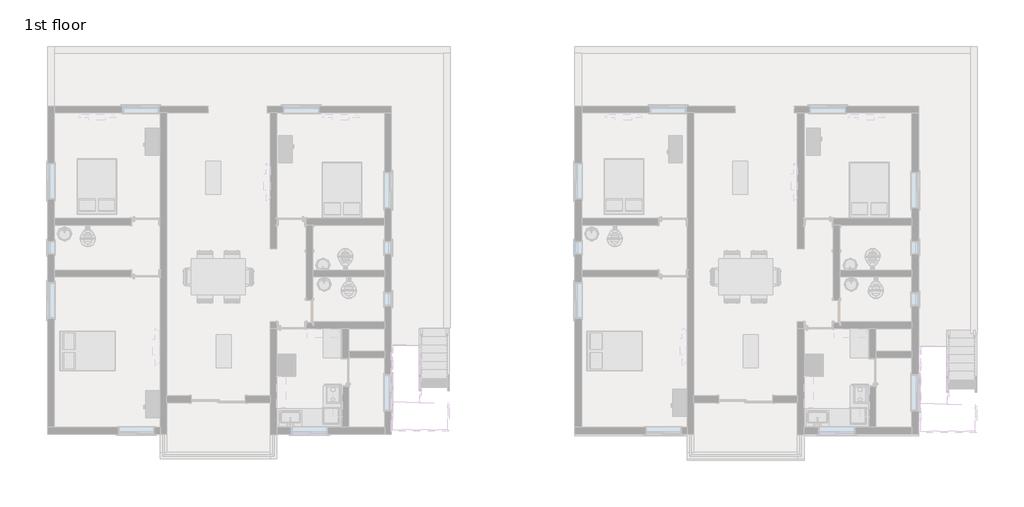
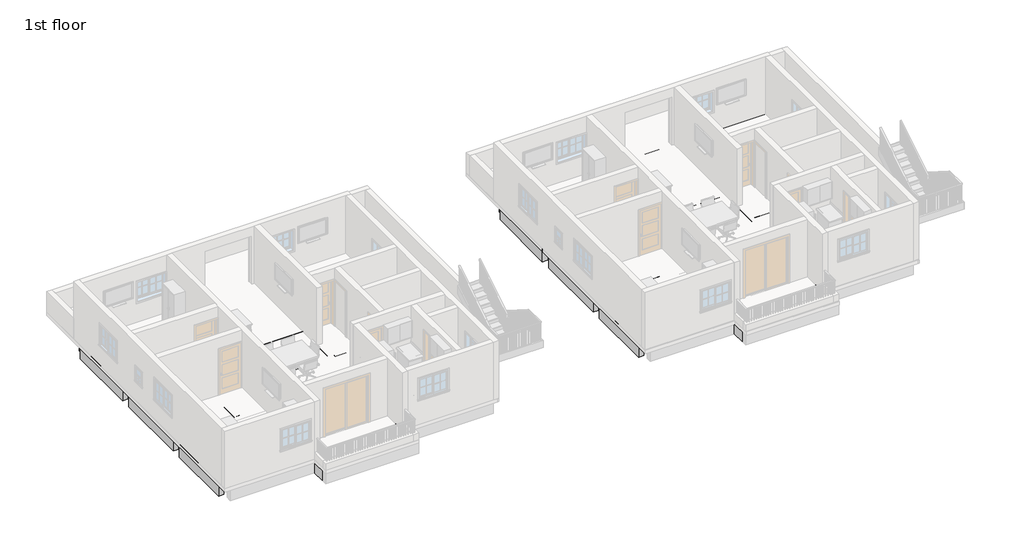
# One storey, part 3 of 8: 30 beams.
"""IFC4 building model written with IfcOpenShell, lengths in millimetres."""

from ifc_helpers import new_model, si_unit, frame, origin, place, context, project, spatial, polyline, outline, extrude, faceted_brep, element, save

model = new_model("IFC4")

# Units and contexts
model_context = context("Model", 3, world=origin())
ifc_project = project(units=[si_unit("LENGTHUNIT", "METRE", prefix="MILLI")], contexts=[model_context])

# Site, building, storey
site = spatial("IfcSite", under=ifc_project)
building = spatial("IfcBuilding", under=site)
storey = spatial("IfcBuildingStorey", under=building, Name="1st floor", Elevation=3810.0)

# Beams
placement = place(None, origin())
element("IfcBeam", 1, ObjectType="Concrete-Rectangular Beam", at=placement, inside=storey, context=model_context, shape_type="Brep", body=[
    faceted_brep([(-16300.5993763, -4148.1064015, 3810.0), (-16071.9993763, -4148.1064015, 3810.0), (-16071.9993763, -1252.5064015, 3810.0), (-16300.5993763, -1252.5064015, 3810.0), (-16300.5993763, -4148.1064015, 3200.4), (-16300.5993763, -1252.5064015, 3200.4), (-16071.9993763, -4148.1064015, 3200.4), (-16071.9993763, -1252.5064015, 3200.4)], [[[0, 1, 2, 3]], [[4, 0, 3, 5]], [[6, 4, 5, 7]], [[1, 6, 7, 2]], [[1, 0, 4, 6]], [[3, 2, 7, 5]]]),
    faceted_brep([(-16300.5993763, 6062.6935985, 3810.0), (-16071.9993763, 6062.6935985, 3810.0), (-16071.9993763, 6062.6935985, 3200.4), (-16300.5993763, 6062.6935985, 3200.4), (-16071.9993763, 2938.4935985, 3810.0), (-16300.5993763, 2938.4935985, 3810.0), (-16300.5993763, 2938.4935985, 3200.4), (-16071.9993763, 2938.4935985, 3200.4)], [[[0, 1, 2, 3]], [[4, 5, 6, 7]], [[1, 0, 5, 4]], [[0, 3, 6, 5]], [[3, 2, 7, 6]], [[2, 1, 4, 7]]]),
    faceted_brep([(-16300.5993763, 2481.2935985, 3810.0), (-16071.9993763, 2481.2935985, 3810.0), (-16071.9993763, 2481.2935985, 3200.4), (-16300.5993763, 2481.2935985, 3200.4), (-16071.9993763, -795.3064015, 3810.0), (-16300.5993763, -795.3064015, 3810.0), (-16300.5993763, -795.3064015, 3200.4), (-16071.9993763, -795.3064015, 3200.4), (-16071.9993763, 728.6935985, 3810.0), (-16071.9993763, 957.2935985, 3810.0), (-16071.9993763, 957.2935985, 3200.4), (-16071.9993763, 728.6935985, 3200.4)], [[[0, 1, 2, 3]], [[4, 5, 6, 7]], [[1, 0, 5, 4, 8, 9]], [[0, 3, 6, 5]], [[3, 2, 10, 11, 7, 6]], [[2, 1, 9, 8, 4, 7, 11, 10]]]),
])
element("IfcBeam", 2, ObjectType="Concrete-Rectangular Beam", at=placement, inside=storey, context=model_context, shape_type="SweptSolid", body=[
    extrude(outline(polyline([(-16071.9993763, 6291.2935985), (-16071.9993763, 6519.8935985), (-12490.5993763, 6519.8935985), (-12490.5993763, 6291.2935985), (-16071.9993763, 6291.2935985)])), frame((0.0, 0.0, 3200.4), z_axis=(0.0, 0.0, 1.0), x_axis=(1.0, 0.0, 0.0)), (0.0, 0.0, 1.0), 609.6),
    extrude(outline(polyline([(-4870.5993763, 6519.8935985), (-4870.5993763, 6291.2935985), (-8528.1993763, 6291.2935985), (-8528.1993763, 6519.8935985), (-4870.5993763, 6519.8935985)])), frame((0.0, 0.0, 3200.4), z_axis=(0.0, 0.0, 1.0), x_axis=(1.0, 0.0, 0.0)), (0.0, 0.0, 1.0), 609.6),
    extrude(outline(polyline([(-12261.9993763, 6291.2935985), (-12261.9993763, 6519.8935985), (-8756.7993763, 6519.8935985), (-8756.7993763, 6291.2935985), (-12261.9993763, 6291.2935985)])), frame((0.0, 0.0, 3200.4), z_axis=(0.0, 0.0, 1.0), x_axis=(1.0, 0.0, 0.0)), (0.0, 0.0, 1.0), 609.6),
])
element("IfcBeam", 3, ObjectType="Concrete-Rectangular Beam", at=placement, inside=storey, context=model_context, shape_type="Brep", body=[
    faceted_brep([(-12261.9993763, -4605.3064015, 3810.0), (-12490.5993763, -4605.3064015, 3810.0), (-12490.5993763, -5214.9064015, 3810.0), (-12261.9993763, -5214.9064015, 3810.0), (-12490.5993763, -4605.3064015, 3200.4), (-12490.5993763, -5214.9064015, 3200.4), (-12261.9993763, -4605.3064015, 3200.4), (-12261.9993763, -5214.9064015, 3200.4)], [[[0, 1, 2, 3]], [[1, 4, 5, 2]], [[4, 6, 7, 5]], [[6, 0, 3, 7]], [[1, 0, 6, 4]], [[3, 2, 5, 7]]]),
    faceted_brep([(-12490.5993763, 6062.6935985, 3810.0), (-12261.9993763, 6062.6935985, 3810.0), (-12261.9993763, 6062.6935985, 3200.4), (-12490.5993763, 6062.6935985, 3200.4), (-12261.9993763, 2938.4935985, 3810.0), (-12490.5993763, 2938.4935985, 3810.0), (-12490.5993763, 2938.4935985, 3200.4), (-12261.9993763, 2938.4935985, 3200.4)], [[[0, 1, 2, 3]], [[4, 5, 6, 7]], [[1, 0, 5, 4]], [[0, 3, 6, 5]], [[3, 2, 7, 6]], [[2, 1, 4, 7]]]),
    faceted_brep([(-12261.9993763, -4148.1064015, 3810.0), (-12490.5993763, -4148.1064015, 3810.0), (-12490.5993763, -4148.1064015, 3200.4), (-12261.9993763, -4148.1064015, 3200.4), (-12490.5993763, -1252.5064015, 3810.0), (-12261.9993763, -1252.5064015, 3810.0), (-12261.9993763, -1252.5064015, 3200.4), (-12490.5993763, -1252.5064015, 3200.4), (-12261.9993763, -3538.5064015, 3810.0), (-12261.9993763, -3309.9064015, 3810.0), (-12261.9993763, -3309.9064015, 3200.4), (-12261.9993763, -3538.5064015, 3200.4)], [[[0, 1, 2, 3]], [[4, 5, 6, 7]], [[1, 0, 8, 9, 5, 4]], [[2, 1, 4, 7]], [[3, 2, 7, 6, 10, 11]], [[0, 3, 11, 10, 6, 5, 9, 8]]]),
    faceted_brep([(-12490.5993763, 2481.2935985, 3810.0), (-12261.9993763, 2481.2935985, 3810.0), (-12261.9993763, 2481.2935985, 3200.4), (-12490.5993763, 2481.2935985, 3200.4), (-12261.9993763, -795.3064015, 3810.0), (-12490.5993763, -795.3064015, 3810.0), (-12490.5993763, -795.3064015, 3200.4), (-12261.9993763, -795.3064015, 3200.4), (-12490.5993763, 957.2935985, 3810.0), (-12490.5993763, 728.6935985, 3810.0), (-12261.9993763, 728.6935985, 3810.0), (-12261.9993763, 957.2935985, 3810.0), (-12490.5993763, 957.2935985, 3200.4), (-12490.5993763, 728.6935985, 3200.4), (-12261.9993763, 957.2935985, 3200.4), (-12261.9993763, 728.6935985, 3200.4)], [[[0, 1, 2, 3]], [[4, 5, 6, 7]], [[1, 0, 8, 9, 5, 4, 10, 11]], [[0, 3, 12, 13, 6, 5, 9, 8]], [[3, 2, 14, 15, 7, 6, 13, 12]], [[2, 1, 11, 10, 4, 7, 15, 14]]]),
])
element("IfcBeam", 4, ObjectType="Concrete-Rectangular Beam", at=placement, inside=storey, context=model_context, shape_type="Brep", body=[
    faceted_brep([(-8528.1993763, 6062.6935985, 3810.0), (-8756.7993763, 6062.6935985, 3810.0), (-8756.7993763, 2938.4935985, 3810.0), (-8528.1993763, 2938.4935985, 3810.0), (-8528.1993763, 6062.6935985, 3200.4), (-8528.1993763, 2938.4935985, 3200.4), (-8756.7993763, 6062.6935985, 3200.4), (-8756.7993763, 2938.4935985, 3200.4)], [[[0, 1, 2, 3]], [[4, 0, 3, 5]], [[6, 4, 5, 7]], [[1, 6, 7, 2]], [[1, 0, 4, 6]], [[3, 2, 7, 5]]]),
    faceted_brep([(-8528.1993763, -5214.9064015, 3810.0), (-8756.7993763, -5214.9064015, 3810.0), (-8756.7993763, -5214.9064015, 3200.4), (-8528.1993763, -5214.9064015, 3200.4), (-8756.7993763, -4605.3064015, 3810.0), (-8528.1993763, -4605.3064015, 3810.0), (-8528.1993763, -4605.3064015, 3200.4), (-8756.7993763, -4605.3064015, 3200.4)], [[[0, 1, 2, 3]], [[4, 5, 6, 7]], [[1, 0, 5, 4]], [[0, 3, 6, 5]], [[3, 2, 7, 6]], [[2, 1, 4, 7]]]),
    faceted_brep([(-8528.1993763, -4148.1064015, 3810.0), (-8756.7993763, -4148.1064015, 3810.0), (-8756.7993763, -4148.1064015, 3200.4), (-8528.1993763, -4148.1064015, 3200.4), (-8756.7993763, -1252.5064015, 3810.0), (-8528.1993763, -1252.5064015, 3810.0), (-8528.1993763, -1252.5064015, 3200.4), (-8756.7993763, -1252.5064015, 3200.4), (-8756.7993763, -3309.9064015, 3810.0), (-8756.7993763, -3538.5064015, 3810.0), (-8756.7993763, -3538.5064015, 3200.4), (-8756.7993763, -3309.9064015, 3200.4)], [[[0, 1, 2, 3]], [[4, 5, 6, 7]], [[1, 0, 5, 4, 8, 9]], [[0, 3, 6, 5]], [[3, 2, 10, 11, 7, 6]], [[2, 1, 9, 8, 4, 7, 11, 10]]]),
    faceted_brep([(-8756.7993763, 2481.2935985, 3810.0), (-8528.1993763, 2481.2935985, 3810.0), (-8528.1993763, 2481.2935985, 3200.4), (-8756.7993763, 2481.2935985, 3200.4), (-8756.7993763, 957.2935985, 3810.0), (-8756.7993763, 728.6935985, 3810.0), (-8756.7993763, -795.3064015, 3810.0), (-8528.1993763, -795.3064015, 3810.0), (-8528.1993763, 728.6935985, 3810.0), (-8528.1993763, 957.2935985, 3810.0), (-8528.1993763, -795.3064015, 3200.4), (-8528.1993763, 728.6935985, 3200.4), (-8528.1993763, 957.2935985, 3200.4), (-8756.7993763, -795.3064015, 3200.4), (-8756.7993763, 728.6935985, 3200.4), (-8756.7993763, 957.2935985, 3200.4)], [[[0, 1, 2, 3]], [[1, 0, 4, 5, 6, 7, 8, 9]], [[2, 1, 9, 8, 7, 10, 11, 12]], [[3, 2, 12, 11, 10, 13, 14, 15]], [[0, 3, 15, 14, 13, 6, 5, 4]], [[7, 6, 13, 10]]]),
])
element("IfcBeam", 5, ObjectType="Concrete-Rectangular Beam", at=placement, inside=storey, context=model_context, shape_type="Brep", body=[
    faceted_brep([(-4870.5993763, -4148.1064015, 3810.0), (-4641.9993763, -4148.1064015, 3810.0), (-4641.9993763, -1023.9064015, 3810.0), (-4870.5993763, -1023.9064015, 3810.0), (-4870.5993763, -1785.9064015, 3810.0), (-4870.5993763, -2014.5064015, 3810.0), (-4870.5993763, -4148.1064015, 3200.4), (-4870.5993763, -1023.9064015, 3200.4), (-4870.5993763, -1785.9064015, 3200.4), (-4870.5993763, -2014.5064015, 3200.4), (-4641.9993763, -4148.1064015, 3200.4), (-4641.9993763, -1023.9064015, 3200.4)], [[[0, 1, 2, 3, 4, 5]], [[6, 0, 5, 4, 3, 7, 8, 9]], [[10, 6, 9, 8, 7, 11]], [[1, 10, 11, 2]], [[1, 0, 6, 10]], [[3, 2, 11, 7]]]),
    faceted_brep([(-4870.5993763, 6062.6935985, 3810.0), (-4641.9993763, 6062.6935985, 3810.0), (-4641.9993763, 6062.6935985, 3200.4), (-4870.5993763, 6062.6935985, 3200.4), (-4641.9993763, 2938.4935985, 3810.0), (-4870.5993763, 2938.4935985, 3810.0), (-4870.5993763, 2938.4935985, 3200.4), (-4641.9993763, 2938.4935985, 3200.4)], [[[0, 1, 2, 3]], [[4, 5, 6, 7]], [[1, 0, 5, 4]], [[0, 3, 6, 5]], [[3, 2, 7, 6]], [[2, 1, 4, 7]]]),
    faceted_brep([(-4870.5993763, 2481.2935985, 3810.0), (-4641.9993763, 2481.2935985, 3810.0), (-4641.9993763, 2481.2935985, 3200.4), (-4870.5993763, 2481.2935985, 3200.4), (-4641.9993763, -566.7064015, 3810.0), (-4870.5993763, -566.7064015, 3810.0), (-4870.5993763, -566.7064015, 3200.4), (-4641.9993763, -566.7064015, 3200.4), (-4870.5993763, 957.2935985, 3810.0), (-4870.5993763, 728.6935985, 3810.0), (-4870.5993763, 957.2935985, 3200.4), (-4870.5993763, 728.6935985, 3200.4)], [[[0, 1, 2, 3]], [[4, 5, 6, 7]], [[1, 0, 8, 9, 5, 4]], [[0, 3, 10, 11, 6, 5, 9, 8]], [[3, 2, 7, 6, 11, 10]], [[2, 1, 4, 7]]]),
])
element("IfcBeam", 6, ObjectType="Concrete-Rectangular Beam", at=placement, inside=storey, context=model_context, shape_type="Brep", body=[
    faceted_brep([(-7308.9993763, 2709.8935985, 3810.0), (-7398.2714156, 2709.8935985, 3810.0), (-7537.5993763, 2709.8935985, 3810.0), (-7537.5993763, 2481.2935985, 3810.0), (-7537.5993763, 957.2935985, 3810.0), (-7537.5993763, 728.6935985, 3810.0), (-7537.5993763, -795.3064015, 3810.0), (-7308.9993763, -795.3064015, 3810.0), (-7308.9993763, 728.6935985, 3810.0), (-7308.9993763, 957.2935985, 3810.0), (-7308.9993763, 2481.2935985, 3810.0), (-7308.9993763, 2709.8935985, 3200.4), (-7308.9993763, -795.3064015, 3200.4), (-7308.9993763, 728.6935985, 3200.4), (-7308.9993763, 957.2935985, 3200.4), (-7308.9993763, 2481.2935985, 3200.4), (-7537.5993763, 2709.8935985, 3200.4), (-7398.2714156, 2709.8935985, 3200.4), (-7537.5993763, -795.3064015, 3200.4), (-7537.5993763, 728.6935985, 3200.4), (-7537.5993763, 957.2935985, 3200.4), (-7537.5993763, 2481.2935985, 3200.4)], [[[0, 1, 2, 3, 4, 5, 6, 7, 8, 9, 10]], [[11, 0, 10, 9, 8, 7, 12, 13, 14, 15]], [[16, 17, 11, 15, 14, 13, 12, 18, 19, 20, 21]], [[2, 16, 21, 20, 19, 18, 6, 5, 4, 3]], [[7, 6, 18, 12]], [[2, 1, 0, 11, 17, 16]]]),
])
element("IfcBeam", 7, ObjectType="Concrete-Rectangular Beam", at=placement, inside=storey, context=model_context, shape_type="SweptSolid", body=[
    extrude(outline(polyline([(-7308.9993763, 2481.2935985), (-7308.9993763, 2709.8935985), (-4870.5993763, 2709.8935985), (-4870.5993763, 2481.2935985), (-7308.9993763, 2481.2935985)])), frame((0.0, 0.0, 3200.4), z_axis=(0.0, 0.0, 1.0), x_axis=(1.0, 0.0, 0.0)), (0.0, 0.0, 1.0), 609.6),
])
element("IfcBeam", 8, ObjectType="Concrete-Rectangular Beam", at=placement, inside=storey, context=model_context, shape_type="SweptSolid", body=[
    extrude(outline(polyline([(-4870.5993763, 957.2935985), (-4870.5993763, 728.6935985), (-7308.9993763, 728.6935985), (-7308.9993763, 957.2935985), (-4870.5993763, 957.2935985)])), frame((0.0, 0.0, 3200.4), z_axis=(0.0, 0.0, 1.0), x_axis=(1.0, 0.0, 0.0)), (0.0, 0.0, 1.0), 609.6),
])
element("IfcBeam", 9, ObjectType="Concrete-Rectangular Beam", at=placement, inside=storey, context=model_context, shape_type="SweptSolid", body=[
    extrude(outline(polyline([(-7537.5993763, 2709.8935985), (-7537.5993763, 2481.2935985), (-8528.1993763, 2481.2935985), (-8528.1993763, 2709.8935985), (-7537.5993763, 2709.8935985)])), frame((0.0, 0.0, 3200.4), z_axis=(0.0, 0.0, 1.0), x_axis=(1.0, 0.0, 0.0)), (0.0, 0.0, 1.0), 609.6),
    extrude(outline(polyline([(-12261.9993763, 2481.2935985), (-12261.9993763, 2709.8935985), (-8756.7993763, 2709.8935985), (-8756.7993763, 2481.2935985), (-12261.9993763, 2481.2935985)])), frame((0.0, 0.0, 3200.4), z_axis=(0.0, 0.0, 1.0), x_axis=(1.0, 0.0, 0.0)), (0.0, 0.0, 1.0), 609.6),
])
element("IfcBeam", 10, ObjectType="Concrete-Rectangular Beam", at=placement, inside=storey, context=model_context, shape_type="Brep", body=[
    faceted_brep([(-13709.7993763, -795.3064015, 3810.0), (-13481.1993763, -795.3064015, 3810.0), (-13481.1993763, 728.6935985, 3810.0), (-13481.1993763, 957.2935985, 3810.0), (-13481.1993763, 2559.3948379, 3810.0), (-13709.7993763, 2562.3306367, 3810.0), (-13709.7993763, 957.2935985, 3810.0), (-13709.7993763, 728.6935985, 3810.0), (-13709.7993763, -795.3064015, 3200.4), (-13709.7993763, 2562.3306367, 3200.4), (-13709.7993763, 957.2935985, 3200.4), (-13709.7993763, 728.6935985, 3200.4), (-13481.1993763, -795.3064015, 3200.4), (-13481.1993763, 2559.3948379, 3200.4), (-13481.1993763, 957.2935985, 3200.4), (-13481.1993763, 728.6935985, 3200.4)], [[[0, 1, 2, 3, 4, 5, 6, 7]], [[8, 0, 7, 6, 5, 9, 10, 11]], [[12, 8, 11, 10, 9, 13, 14, 15]], [[1, 12, 15, 14, 13, 4, 3, 2]], [[1, 0, 8, 12]], [[5, 4, 13, 9]]]),
])
element("IfcBeam", 11, ObjectType="Concrete-Rectangular Beam", at=placement, inside=storey, context=model_context, shape_type="SweptSolid", body=[
    extrude(outline(polyline([(-16071.9993763, 728.6935985), (-16071.9993763, 957.2935985), (-13709.7993763, 957.2935985), (-13709.7993763, 728.6935985), (-16071.9993763, 728.6935985)])), frame((0.0, 0.0, 3200.4), z_axis=(0.0, 0.0, 1.0), x_axis=(1.0, 0.0, 0.0)), (0.0, 0.0, 1.0), 609.6),
])
element("IfcBeam", 12, ObjectType="Concrete-Rectangular Beam", at=placement, inside=storey, context=model_context, shape_type="SweptSolid", body=[
    extrude(outline(polyline([(-12490.5993763, 957.2935985), (-12490.5993763, 728.6935985), (-13481.1993763, 728.6935985), (-13481.1993763, 957.2935985), (-12490.5993763, 957.2935985)])), frame((0.0, 0.0, 3200.4), z_axis=(0.0, 0.0, 1.0), x_axis=(1.0, 0.0, 0.0)), (0.0, 0.0, 1.0), 609.6),
])
element("IfcBeam", 13, ObjectType="Concrete-Rectangular Beam", at=placement, inside=storey, context=model_context, shape_type="SweptSolid", body=[
    extrude(outline(polyline([(-12261.9993763, 728.6935985), (-12261.9993763, 957.2935985), (-8756.7993763, 957.2935985), (-8756.7993763, 728.6935985), (-12261.9993763, 728.6935985)])), frame((0.0, 0.0, 3200.4), z_axis=(0.0, 0.0, 1.0), x_axis=(1.0, 0.0, 0.0)), (0.0, 0.0, 1.0), 609.6),
    extrude(outline(polyline([(-7537.5993763, 957.2935985), (-7537.5993763, 728.6935985), (-8528.1993763, 728.6935985), (-8528.1993763, 957.2935985), (-7537.5993763, 957.2935985)])), frame((0.0, 0.0, 3200.4), z_axis=(0.0, 0.0, 1.0), x_axis=(1.0, 0.0, 0.0)), (0.0, 0.0, 1.0), 609.6),
])
element("IfcBeam", 14, ObjectType="Concrete-Rectangular Beam", at=placement, inside=storey, context=model_context, shape_type="Brep", body=[
    faceted_brep([(-12490.5993763, 2546.6730431, 3810.0), (-12490.5993763, 2775.2918938, 3810.0), (-16071.9993763, 2821.286075, 3810.0), (-16071.9993763, 2592.6672243, 3810.0), (-13709.7993763, 2562.3306367, 3810.0), (-13481.1993763, 2559.3948379, 3810.0), (-12490.5993763, 2775.2918938, 3200.4), (-16071.9993763, 2821.286075, 3200.4), (-12490.5993763, 2546.6730431, 3200.4), (-13481.1993763, 2559.3948379, 3200.4), (-13709.7993763, 2562.3306367, 3200.4), (-16071.9993763, 2592.6672243, 3200.4)], [[[0, 1, 2, 3, 4, 5]], [[1, 6, 7, 2]], [[6, 8, 9, 10, 11, 7]], [[8, 0, 5, 4, 3, 11, 10, 9]], [[1, 0, 8, 6]], [[3, 2, 7, 11]]]),
    faceted_brep([(-12261.9993763, 2709.8935985, 3810.0), (-12261.9993763, 2709.8935985, 3200.4), (-8756.7993763, 2709.8935985, 3200.4), (-8756.7993763, 2709.8935985, 3810.0), (-12261.9993763, 2772.356095, 3810.0), (-12261.9993763, 2772.356095, 3200.4), (-8756.7993763, 2727.3405134, 3810.0), (-8756.7993763, 2727.3405134, 3200.4)], [[[0, 1, 2, 3]], [[0, 4, 5, 1]], [[4, 0, 3, 6]], [[5, 4, 6, 7]], [[1, 5, 7, 2]], [[3, 2, 7, 6]]]),
    faceted_brep([(-8528.1993763, 2709.8935985, 3200.4), (-8528.1993763, 2709.8935985, 3810.0), (-8528.1993763, 2724.4047146, 3810.0), (-8528.1993763, 2724.4047146, 3200.4), (-7398.2714156, 2709.8935985, 3200.4), (-7398.2714156, 2709.8935985, 3810.0), (-7537.5993763, 2709.8935985, 3810.0), (-7537.5993763, 2709.8935985, 3200.4)], [[[0, 1, 2, 3]], [[4, 5, 6, 1, 0, 7]], [[1, 6, 5, 2]], [[5, 4, 3, 2]], [[4, 7, 0, 3]]]),
])
element("IfcBeam", 15, ObjectType="Concrete-Rectangular Beam", at=placement, inside=storey, context=model_context, shape_type="Brep", body=[
    faceted_brep([(1573.9761273, -4148.1064015, 3810.0), (1802.5761273, -4148.1064015, 3810.0), (1802.5761273, -1252.5064015, 3810.0), (1573.9761273, -1252.5064015, 3810.0), (1573.9761273, -4148.1064015, 3200.4), (1573.9761273, -1252.5064015, 3200.4), (1802.5761273, -4148.1064015, 3200.4), (1802.5761273, -1252.5064015, 3200.4)], [[[0, 1, 2, 3]], [[4, 0, 3, 5]], [[6, 4, 5, 7]], [[1, 6, 7, 2]], [[1, 0, 4, 6]], [[3, 2, 7, 5]]]),
    faceted_brep([(1573.9761273, 6062.6935985, 3810.0), (1802.5761273, 6062.6935985, 3810.0), (1802.5761273, 6062.6935985, 3200.4), (1573.9761273, 6062.6935985, 3200.4), (1802.5761273, 2938.4935985, 3810.0), (1573.9761273, 2938.4935985, 3810.0), (1573.9761273, 2938.4935985, 3200.4), (1802.5761273, 2938.4935985, 3200.4)], [[[0, 1, 2, 3]], [[4, 5, 6, 7]], [[1, 0, 5, 4]], [[0, 3, 6, 5]], [[3, 2, 7, 6]], [[2, 1, 4, 7]]]),
    faceted_brep([(1573.9761273, 2481.2935985, 3810.0), (1802.5761273, 2481.2935985, 3810.0), (1802.5761273, 2481.2935985, 3200.4), (1573.9761273, 2481.2935985, 3200.4), (1802.5761273, -795.3064015, 3810.0), (1573.9761273, -795.3064015, 3810.0), (1573.9761273, -795.3064015, 3200.4), (1802.5761273, -795.3064015, 3200.4), (1802.5761273, 728.6935985, 3810.0), (1802.5761273, 957.2935985, 3810.0), (1802.5761273, 957.2935985, 3200.4), (1802.5761273, 728.6935985, 3200.4)], [[[0, 1, 2, 3]], [[4, 5, 6, 7]], [[1, 0, 5, 4, 8, 9]], [[0, 3, 6, 5]], [[3, 2, 10, 11, 7, 6]], [[2, 1, 9, 8, 4, 7, 11, 10]]]),
])
element("IfcBeam", 16, ObjectType="Concrete-Rectangular Beam", at=placement, inside=storey, context=model_context, shape_type="SweptSolid", body=[
    extrude(outline(polyline([(1802.5761273, 6291.2935985), (1802.5761273, 6519.8935985), (5383.9761273, 6519.8935985), (5383.9761273, 6291.2935985), (1802.5761273, 6291.2935985)])), frame((0.0, 0.0, 3200.4), z_axis=(0.0, 0.0, 1.0), x_axis=(1.0, 0.0, 0.0)), (0.0, 0.0, 1.0), 609.6),
    extrude(outline(polyline([(13003.9761273, 6519.8935985), (13003.9761273, 6291.2935985), (9346.3761273, 6291.2935985), (9346.3761273, 6519.8935985), (13003.9761273, 6519.8935985)])), frame((0.0, 0.0, 3200.4), z_axis=(0.0, 0.0, 1.0), x_axis=(1.0, 0.0, 0.0)), (0.0, 0.0, 1.0), 609.6),
    extrude(outline(polyline([(5612.5761273, 6291.2935985), (5612.5761273, 6519.8935985), (9117.7761273, 6519.8935985), (9117.7761273, 6291.2935985), (5612.5761273, 6291.2935985)])), frame((0.0, 0.0, 3200.4), z_axis=(0.0, 0.0, 1.0), x_axis=(1.0, 0.0, 0.0)), (0.0, 0.0, 1.0), 609.6),
])
element("IfcBeam", 17, ObjectType="Concrete-Rectangular Beam", at=placement, inside=storey, context=model_context, shape_type="Brep", body=[
    faceted_brep([(5612.5761273, -4605.3064015, 3810.0), (5383.9761273, -4605.3064015, 3810.0), (5383.9761273, -5214.9064015, 3810.0), (5612.5761273, -5214.9064015, 3810.0), (5383.9761273, -4605.3064015, 3200.4), (5383.9761273, -5214.9064015, 3200.4), (5612.5761273, -4605.3064015, 3200.4), (5612.5761273, -5214.9064015, 3200.4)], [[[0, 1, 2, 3]], [[1, 4, 5, 2]], [[4, 6, 7, 5]], [[6, 0, 3, 7]], [[1, 0, 6, 4]], [[3, 2, 5, 7]]]),
    faceted_brep([(5383.9761273, 6062.6935985, 3810.0), (5612.5761273, 6062.6935985, 3810.0), (5612.5761273, 6062.6935985, 3200.4), (5383.9761273, 6062.6935985, 3200.4), (5612.5761273, 2938.4935985, 3810.0), (5383.9761273, 2938.4935985, 3810.0), (5383.9761273, 2938.4935985, 3200.4), (5612.5761273, 2938.4935985, 3200.4)], [[[0, 1, 2, 3]], [[4, 5, 6, 7]], [[1, 0, 5, 4]], [[0, 3, 6, 5]], [[3, 2, 7, 6]], [[2, 1, 4, 7]]]),
    faceted_brep([(5612.5761273, -4148.1064015, 3810.0), (5383.9761273, -4148.1064015, 3810.0), (5383.9761273, -4148.1064015, 3200.4), (5612.5761273, -4148.1064015, 3200.4), (5383.9761273, -1252.5064015, 3810.0), (5612.5761273, -1252.5064015, 3810.0), (5612.5761273, -1252.5064015, 3200.4), (5383.9761273, -1252.5064015, 3200.4), (5612.5761273, -3538.5064015, 3810.0), (5612.5761273, -3309.9064015, 3810.0), (5612.5761273, -3309.9064015, 3200.4), (5612.5761273, -3538.5064015, 3200.4)], [[[0, 1, 2, 3]], [[4, 5, 6, 7]], [[1, 0, 8, 9, 5, 4]], [[2, 1, 4, 7]], [[3, 2, 7, 6, 10, 11]], [[0, 3, 11, 10, 6, 5, 9, 8]]]),
    faceted_brep([(5383.9761273, 2481.2935985, 3810.0), (5612.5761273, 2481.2935985, 3810.0), (5612.5761273, 2481.2935985, 3200.4), (5383.9761273, 2481.2935985, 3200.4), (5612.5761273, -795.3064015, 3810.0), (5383.9761273, -795.3064015, 3810.0), (5383.9761273, -795.3064015, 3200.4), (5612.5761273, -795.3064015, 3200.4), (5383.9761273, 957.2935985, 3810.0), (5383.9761273, 728.6935985, 3810.0), (5612.5761273, 728.6935985, 3810.0), (5612.5761273, 957.2935985, 3810.0), (5383.9761273, 957.2935985, 3200.4), (5383.9761273, 728.6935985, 3200.4), (5612.5761273, 957.2935985, 3200.4), (5612.5761273, 728.6935985, 3200.4)], [[[0, 1, 2, 3]], [[4, 5, 6, 7]], [[1, 0, 8, 9, 5, 4, 10, 11]], [[0, 3, 12, 13, 6, 5, 9, 8]], [[3, 2, 14, 15, 7, 6, 13, 12]], [[2, 1, 11, 10, 4, 7, 15, 14]]]),
])
element("IfcBeam", 18, ObjectType="Concrete-Rectangular Beam", at=placement, inside=storey, context=model_context, shape_type="Brep", body=[
    faceted_brep([(9346.3761273, 6062.6935985, 3810.0), (9117.7761273, 6062.6935985, 3810.0), (9117.7761273, 2938.4935985, 3810.0), (9346.3761273, 2938.4935985, 3810.0), (9346.3761273, 6062.6935985, 3200.4), (9346.3761273, 2938.4935985, 3200.4), (9117.7761273, 6062.6935985, 3200.4), (9117.7761273, 2938.4935985, 3200.4)], [[[0, 1, 2, 3]], [[4, 0, 3, 5]], [[6, 4, 5, 7]], [[1, 6, 7, 2]], [[1, 0, 4, 6]], [[3, 2, 7, 5]]]),
    faceted_brep([(9346.3761273, -5214.9064015, 3810.0), (9117.7761273, -5214.9064015, 3810.0), (9117.7761273, -5214.9064015, 3200.4), (9346.3761273, -5214.9064015, 3200.4), (9117.7761273, -4605.3064015, 3810.0), (9346.3761273, -4605.3064015, 3810.0), (9346.3761273, -4605.3064015, 3200.4), (9117.7761273, -4605.3064015, 3200.4)], [[[0, 1, 2, 3]], [[4, 5, 6, 7]], [[1, 0, 5, 4]], [[6, 5, 0, 3]], [[3, 2, 7, 6]], [[2, 1, 4, 7]]]),
    faceted_brep([(9346.3761273, -4148.1064015, 3810.0), (9117.7761273, -4148.1064015, 3810.0), (9117.7761273, -4148.1064015, 3200.4), (9346.3761273, -4148.1064015, 3200.4), (9117.7761273, -1252.5064015, 3810.0), (9346.3761273, -1252.5064015, 3810.0), (9346.3761273, -1252.5064015, 3200.4), (9117.7761273, -1252.5064015, 3200.4), (9117.7761273, -3309.9064015, 3810.0), (9117.7761273, -3538.5064015, 3810.0), (9117.7761273, -3538.5064015, 3200.4), (9117.7761273, -3309.9064015, 3200.4)], [[[0, 1, 2, 3]], [[4, 5, 6, 7]], [[1, 0, 5, 4, 8, 9]], [[0, 3, 6, 5]], [[3, 2, 10, 11, 7, 6]], [[2, 1, 9, 8, 4, 7, 11, 10]]]),
    faceted_brep([(9117.7761273, 2481.2935985, 3810.0), (9346.3761273, 2481.2935985, 3810.0), (9346.3761273, 2481.2935985, 3200.4), (9117.7761273, 2481.2935985, 3200.4), (9117.7761273, 957.2935985, 3810.0), (9117.7761273, 728.6935985, 3810.0), (9117.7761273, -795.3064015, 3810.0), (9346.3761273, -795.3064015, 3810.0), (9346.3761273, 728.6935985, 3810.0), (9346.3761273, 957.2935985, 3810.0), (9346.3761273, -795.3064015, 3200.4), (9346.3761273, 728.6935985, 3200.4), (9346.3761273, 957.2935985, 3200.4), (9117.7761273, -795.3064015, 3200.4), (9117.7761273, 728.6935985, 3200.4), (9117.7761273, 957.2935985, 3200.4)], [[[0, 1, 2, 3]], [[1, 0, 4, 5, 6, 7, 8, 9]], [[2, 1, 9, 8, 7, 10, 11, 12]], [[3, 2, 12, 11, 10, 13, 14, 15]], [[0, 3, 15, 14, 13, 6, 5, 4]], [[7, 6, 13, 10]]]),
])
element("IfcBeam", 19, ObjectType="Concrete-Rectangular Beam", at=placement, inside=storey, context=model_context, shape_type="Brep", body=[
    faceted_brep([(13003.9761273, -4148.1064015, 3810.0), (13232.5761273, -4148.1064015, 3810.0), (13232.5761273, -1023.9064015, 3810.0), (13003.9761273, -1023.9064015, 3810.0), (13003.9761273, -1785.9064015, 3810.0), (13003.9761273, -2014.5064015, 3810.0), (13003.9761273, -4148.1064015, 3200.4), (13003.9761273, -1023.9064015, 3200.4), (13003.9761273, -1785.9064015, 3200.4), (13003.9761273, -2014.5064015, 3200.4), (13232.5761273, -4148.1064015, 3200.4), (13232.5761273, -1023.9064015, 3200.4)], [[[0, 1, 2, 3, 4, 5]], [[6, 0, 5, 4, 3, 7, 8, 9]], [[10, 6, 9, 8, 7, 11]], [[1, 10, 11, 2]], [[1, 0, 6, 10]], [[3, 2, 11, 7]]]),
    faceted_brep([(13003.9761273, 6062.6935985, 3810.0), (13232.5761273, 6062.6935985, 3810.0), (13232.5761273, 6062.6935985, 3200.4), (13003.9761273, 6062.6935985, 3200.4), (13232.5761273, 2938.4935985, 3810.0), (13003.9761273, 2938.4935985, 3810.0), (13003.9761273, 2938.4935985, 3200.4), (13232.5761273, 2938.4935985, 3200.4)], [[[0, 1, 2, 3]], [[4, 5, 6, 7]], [[1, 0, 5, 4]], [[0, 3, 6, 5]], [[3, 2, 7, 6]], [[2, 1, 4, 7]]]),
    faceted_brep([(13003.9761273, 2481.2935985, 3810.0), (13232.5761273, 2481.2935985, 3810.0), (13232.5761273, 2481.2935985, 3200.4), (13003.9761273, 2481.2935985, 3200.4), (13232.5761273, -566.7064015, 3810.0), (13003.9761273, -566.7064015, 3810.0), (13003.9761273, -566.7064015, 3200.4), (13232.5761273, -566.7064015, 3200.4), (13003.9761273, 957.2935985, 3810.0), (13003.9761273, 728.6935985, 3810.0), (13003.9761273, 957.2935985, 3200.4), (13003.9761273, 728.6935985, 3200.4)], [[[0, 1, 2, 3]], [[4, 5, 6, 7]], [[1, 0, 8, 9, 5, 4]], [[0, 3, 10, 11, 6, 5, 9, 8]], [[3, 2, 7, 6, 11, 10]], [[2, 1, 4, 7]]]),
])
element("IfcBeam", 20, ObjectType="Concrete-Rectangular Beam", at=placement, inside=storey, context=model_context, shape_type="Brep", body=[
    faceted_brep([(9346.3761273, -795.3064015, 3810.0), (9346.3761273, -1023.9064015, 3810.0), (11556.1761273, -1023.9064015, 3810.0), (11784.7761273, -1023.9064015, 3810.0), (13003.9761273, -1023.9064015, 3810.0), (13003.9761273, -795.3064015, 3810.0), (10565.5761273, -795.3064015, 3810.0), (10336.9761273, -795.3064015, 3810.0), (9346.3761273, -795.3064015, 3200.4), (13003.9761273, -795.3064015, 3200.4), (10565.5761273, -795.3064015, 3200.4), (10336.9761273, -795.3064015, 3200.4), (9346.3761273, -1023.9064015, 3200.4), (13003.9761273, -1023.9064015, 3200.4), (11784.7761273, -1023.9064015, 3200.4), (11556.1761273, -1023.9064015, 3200.4)], [[[0, 1, 2, 3, 4, 5, 6, 7]], [[8, 0, 7, 6, 5, 9, 10, 11]], [[12, 8, 11, 10, 9, 13, 14, 15]], [[1, 12, 15, 14, 13, 4, 3, 2]], [[1, 0, 8, 12]], [[5, 4, 13, 9]]]),
])
element("IfcBeam", 21, ObjectType="Concrete-Rectangular Beam", at=placement, inside=storey, context=model_context, shape_type="SweptSolid", body=[
    extrude(outline(polyline([(13003.9761273, -1785.9064015), (13003.9761273, -2014.5064015), (11784.7761273, -2014.5064015), (11784.7761273, -1785.9064015), (13003.9761273, -1785.9064015)])), frame((0.0, 0.0, 3200.4), z_axis=(0.0, 0.0, 1.0), x_axis=(1.0, 0.0, 0.0)), (0.0, 0.0, 1.0), 609.6),
])
element("IfcBeam", 22, ObjectType="Concrete-Rectangular Beam", at=placement, inside=storey, context=model_context, shape_type="Brep", body=[
    faceted_brep([(10565.5761273, 2709.8935985, 3810.0), (10476.304088, 2709.8935985, 3810.0), (10336.9761273, 2709.8935985, 3810.0), (10336.9761273, 2483.0640691, 3810.0), (10336.9761273, 2481.2935985, 3810.0), (10336.9761273, 957.2935985, 3810.0), (10336.9761273, 728.6935985, 3810.0), (10336.9761273, -795.3064015, 3810.0), (10565.5761273, -795.3064015, 3810.0), (10565.5761273, 728.6935985, 3810.0), (10565.5761273, 957.2935985, 3810.0), (10565.5761273, 2481.2935985, 3810.0), (10565.5761273, 2709.8935985, 3200.4), (10565.5761273, -795.3064015, 3200.4), (10565.5761273, 728.6935985, 3200.4), (10565.5761273, 957.2935985, 3200.4), (10565.5761273, 2481.2935985, 3200.4), (10336.9761273, 2709.8935985, 3200.4), (10476.304088, 2709.8935985, 3200.4), (10336.9761273, -795.3064015, 3200.4), (10336.9761273, 728.6935985, 3200.4), (10336.9761273, 957.2935985, 3200.4), (10336.9761273, 2481.2935985, 3200.4), (10336.9761273, 2483.0640691, 3200.4)], [[[0, 1, 2, 3, 4, 5, 6, 7, 8, 9, 10, 11]], [[12, 0, 11, 10, 9, 8, 13, 14, 15, 16]], [[17, 18, 12, 16, 15, 14, 13, 19, 20, 21, 22, 23]], [[2, 17, 23, 22, 21, 20, 19, 7, 6, 5, 4, 3]], [[8, 7, 19, 13]], [[2, 1, 0, 12, 18, 17]]]),
])
element("IfcBeam", 23, ObjectType="Concrete-Rectangular Beam", at=placement, inside=storey, context=model_context, shape_type="SweptSolid", body=[
    extrude(outline(polyline([(10565.5761273, 2481.2935985), (10565.5761273, 2709.8935985), (13003.9761273, 2709.8935985), (13003.9761273, 2481.2935985), (10565.5761273, 2481.2935985)])), frame((0.0, 0.0, 3200.4), z_axis=(0.0, 0.0, 1.0), x_axis=(1.0, 0.0, 0.0)), (0.0, 0.0, 1.0), 609.6),
])
element("IfcBeam", 24, ObjectType="Concrete-Rectangular Beam", at=placement, inside=storey, context=model_context, shape_type="SweptSolid", body=[
    extrude(outline(polyline([(13003.9761273, 957.2935985), (13003.9761273, 728.6935985), (10565.5761273, 728.6935985), (10565.5761273, 957.2935985), (13003.9761273, 957.2935985)])), frame((0.0, 0.0, 3200.4), z_axis=(0.0, 0.0, 1.0), x_axis=(1.0, 0.0, 0.0)), (0.0, 0.0, 1.0), 609.6),
])
element("IfcBeam", 25, ObjectType="Concrete-Rectangular Beam", at=placement, inside=storey, context=model_context, shape_type="SweptSolid", body=[
    extrude(outline(polyline([(5612.5761273, 2481.2935985), (5612.5761273, 2709.8935985), (9117.7761273, 2709.8935985), (9117.7761273, 2481.2935985), (5612.5761273, 2481.2935985)])), frame((0.0, 0.0, 3200.4), z_axis=(0.0, 0.0, 1.0), x_axis=(1.0, 0.0, 0.0)), (0.0, 0.0, 1.0), 609.6),
    extrude(outline(polyline([(10336.9761273, 2709.8935985), (10336.9761273, 2481.2935985), (9346.3761273, 2481.2935985), (9346.3761273, 2709.8935985), (10336.9761273, 2709.8935985)])), frame((0.0, 0.0, 3200.4), z_axis=(0.0, 0.0, 1.0), x_axis=(1.0, 0.0, 0.0)), (0.0, 0.0, 1.0), 609.6),
])
element("IfcBeam", 26, ObjectType="Concrete-Rectangular Beam", at=placement, inside=storey, context=model_context, shape_type="Brep", body=[
    faceted_brep([(4164.7761273, -795.3064015, 3810.0), (4393.3761273, -795.3064015, 3810.0), (4393.3761273, 728.6935985, 3810.0), (4393.3761273, 957.2935985, 3810.0), (4393.3761273, 2559.3948379, 3810.0), (4164.7761273, 2562.3306367, 3810.0), (4164.7761273, 957.2935985, 3810.0), (4164.7761273, 728.6935985, 3810.0), (4164.7761273, -795.3064015, 3200.4), (4164.7761273, 2562.3306367, 3200.4), (4164.7761273, 957.2935985, 3200.4), (4164.7761273, 728.6935985, 3200.4), (4393.3761273, -795.3064015, 3200.4), (4393.3761273, 2559.3948379, 3200.4), (4393.3761273, 957.2935985, 3200.4), (4393.3761273, 728.6935985, 3200.4)], [[[0, 1, 2, 3, 4, 5, 6, 7]], [[8, 0, 7, 6, 5, 9, 10, 11]], [[12, 8, 11, 10, 9, 13, 14, 15]], [[1, 12, 15, 14, 13, 4, 3, 2]], [[1, 0, 8, 12]], [[5, 4, 13, 9]]]),
])
element("IfcBeam", 27, ObjectType="Concrete-Rectangular Beam", at=placement, inside=storey, context=model_context, shape_type="SweptSolid", body=[
    extrude(outline(polyline([(1802.5761273, 728.6935985), (1802.5761273, 957.2935985), (4164.7761273, 957.2935985), (4164.7761273, 728.6935985), (1802.5761273, 728.6935985)])), frame((0.0, 0.0, 3200.4), z_axis=(0.0, 0.0, 1.0), x_axis=(1.0, 0.0, 0.0)), (0.0, 0.0, 1.0), 609.6),
])
element("IfcBeam", 28, ObjectType="Concrete-Rectangular Beam", at=placement, inside=storey, context=model_context, shape_type="SweptSolid", body=[
    extrude(outline(polyline([(5383.9761273, 957.2935985), (5383.9761273, 728.6935985), (4393.3761273, 728.6935985), (4393.3761273, 957.2935985), (5383.9761273, 957.2935985)])), frame((0.0, 0.0, 3200.4), z_axis=(0.0, 0.0, 1.0), x_axis=(1.0, 0.0, 0.0)), (0.0, 0.0, 1.0), 609.6),
])
element("IfcBeam", 29, ObjectType="Concrete-Rectangular Beam", at=placement, inside=storey, context=model_context, shape_type="SweptSolid", body=[
    extrude(outline(polyline([(5612.5761273, 728.6935985), (5612.5761273, 957.2935985), (9117.7761273, 957.2935985), (9117.7761273, 728.6935985), (5612.5761273, 728.6935985)])), frame((0.0, 0.0, 3200.4), z_axis=(0.0, 0.0, 1.0), x_axis=(1.0, 0.0, 0.0)), (0.0, 0.0, 1.0), 609.6),
    extrude(outline(polyline([(10336.9761273, 957.2935985), (10336.9761273, 728.6935985), (9346.3761273, 728.6935985), (9346.3761273, 957.2935985), (10336.9761273, 957.2935985)])), frame((0.0, 0.0, 3200.4), z_axis=(0.0, 0.0, 1.0), x_axis=(1.0, 0.0, 0.0)), (0.0, 0.0, 1.0), 609.6),
])
element("IfcBeam", 30, ObjectType="Concrete-Rectangular Beam", at=placement, inside=storey, context=model_context, shape_type="Brep", body=[
    faceted_brep([(5383.9761273, 2546.6730431, 3810.0), (5383.9761273, 2775.2918938, 3810.0), (1802.5761273, 2821.286075, 3810.0), (1802.5761273, 2592.6672243, 3810.0), (4164.7761273, 2562.3306367, 3810.0), (4393.3761273, 2559.3948379, 3810.0), (5383.9761273, 2775.2918938, 3200.4), (1802.5761273, 2821.286075, 3200.4), (5383.9761273, 2546.6730431, 3200.4), (4393.3761273, 2559.3948379, 3200.4), (4164.7761273, 2562.3306367, 3200.4), (1802.5761273, 2592.6672243, 3200.4)], [[[0, 1, 2, 3, 4, 5]], [[1, 6, 7, 2]], [[6, 8, 9, 10, 11, 7]], [[8, 0, 5, 4, 3, 11, 10, 9]], [[1, 0, 8, 6]], [[3, 2, 7, 11]]]),
    faceted_brep([(10336.9761273, 2709.8935985, 3810.0), (10336.9761273, 2483.0640691, 3810.0), (10336.9761273, 2483.0640691, 3200.4), (10336.9761273, 2709.8935985, 3200.4), (9346.3761273, 2495.7858639, 3810.0), (9346.3761273, 2724.4047146, 3810.0), (9346.3761273, 2724.4047146, 3200.4), (9346.3761273, 2495.7858639, 3200.4), (10476.304088, 2709.8935985, 3810.0), (10476.304088, 2709.8935985, 3200.4)], [[[0, 1, 2, 3]], [[4, 5, 6, 7]], [[1, 0, 8, 5, 4]], [[8, 9, 6, 5]], [[3, 2, 7, 6, 9]], [[2, 1, 4, 7]], [[0, 3, 9, 8]]]),
    faceted_brep([(5612.5761273, 2543.7372443, 3810.0), (5612.5761273, 2772.356095, 3810.0), (5612.5761273, 2772.356095, 3200.4), (5612.5761273, 2543.7372443, 3200.4), (9117.7761273, 2498.7216627, 3810.0), (9117.7761273, 2727.3405134, 3810.0), (9117.7761273, 2727.3405134, 3200.4), (9117.7761273, 2498.7216627, 3200.4)], [[[0, 1, 2, 3]], [[1, 0, 4, 5]], [[2, 1, 5, 6]], [[3, 2, 6, 7]], [[5, 4, 7, 6]], [[0, 3, 7, 4]]]),
])

save(model, "model.ifc")

# Revit data of these elements
# Type "Concrete-Rectangular Beam"
#   Assembly Code = "B10"
#   Length [instance default] = 5' - 0"
#   b = 0' - 9"
#   h = 2' - 0"
#   Structural Material [instance default] = Concrete, Cast-in-Place gray
# Elements 1, 2, 3, 4, 5, 6, 7, 8, 9, 10, 11, 12, 13, 14, 15, 16, 17, 18, 19, 20, 21, 22, 23, 24, 25, 26, 27, 28, 29, 30 (IfcBeam, "Concrete-Rectangular Beam")
#   Structural Material = Concrete, Cast-in-Place gray
#   Phase Created = New Construction
#   Materials on its faces: "Concrete, Cast-in-Place gray"
# Materials
#   "Concrete, Cast-in-Place gray": class "Concrete", colour RGB 192 192 192, transparency 0, Description = "Cast-in-place concrete", Cost = 0
